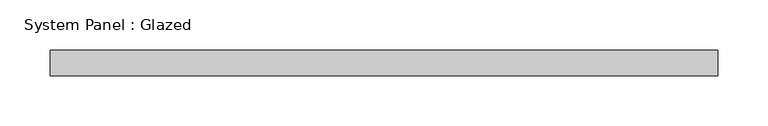
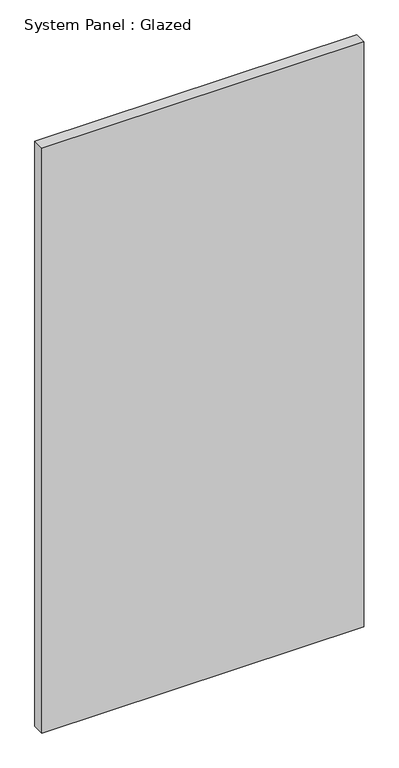
"""IFC4 building model written with IfcOpenShell, lengths in millimetres: plate geometry, System Panel : Glazed."""

from ifc_helpers import new_model, si_unit, origin, origin_with_axes, place, context, project, spatial, polyline, outline, extrude, source, transform, mapped, element, save


def system_panel_glazed_dcc89d10(model_context):
    return source(origin(), model_context, "Body", "SweptSolid", [
        extrude(outline(polyline([(333.375, 19.05), (-333.375, 19.05), (-333.375, 44.45), (333.375, 44.45), (333.375, 19.05)])), origin_with_axes(), (0.0, 0.0, 1.0), 1281.1788335),
    ])


if __name__ == "__main__":
    model = new_model("IFC4")
    model_context = context("Model", 3, world=origin())
    ifc_project = project(units=[si_unit("LENGTHUNIT", "METRE", prefix="MILLI")], contexts=[model_context])
    site = spatial("IfcSite", under=ifc_project)
    building = spatial("IfcBuilding", under=site)
    placement = place(None, origin())
    system_panel_glazed_shape = system_panel_glazed_dcc89d10(model_context)
    element("IfcPlate", 1, ObjectType="System Panel : Glazed", at=placement, inside=building, context=model_context, shape_type="MappedRepresentation", body=[
        mapped(system_panel_glazed_shape, transform((0.0, 0.0, 0.0), x_axis=(1.0, 0.0, 0.0), y_axis=(0.0, 1.0, 0.0), z_axis=(0.0, 0.0, 1.0))),
    ])
    save(model, "model.ifc")

# Revit data of these elements
# Type "System Panel : Glazed"
#   Construction Type Id = "GSP4R"
#   Analytic Construction = "1/8 in Pilkington single glazing"
#   Visual Light Transmittance = 0.9
#   Solar Heat Gain Coefficient = 0.86
#   Heat Transfer Coefficient (U) = 1.18115 BTU/(h·ft²·°F)
#   Define Thermal Properties by = 1
# Element 1 (IfcPlate, "System Panel : Glazed")
#   Materials on its faces: "Glass"
# Materials
#   "Glass": class "Glass", colour RGB 0 128 192, transparency 0.75, Description = "Soda Lime Glass", Cost = 0
